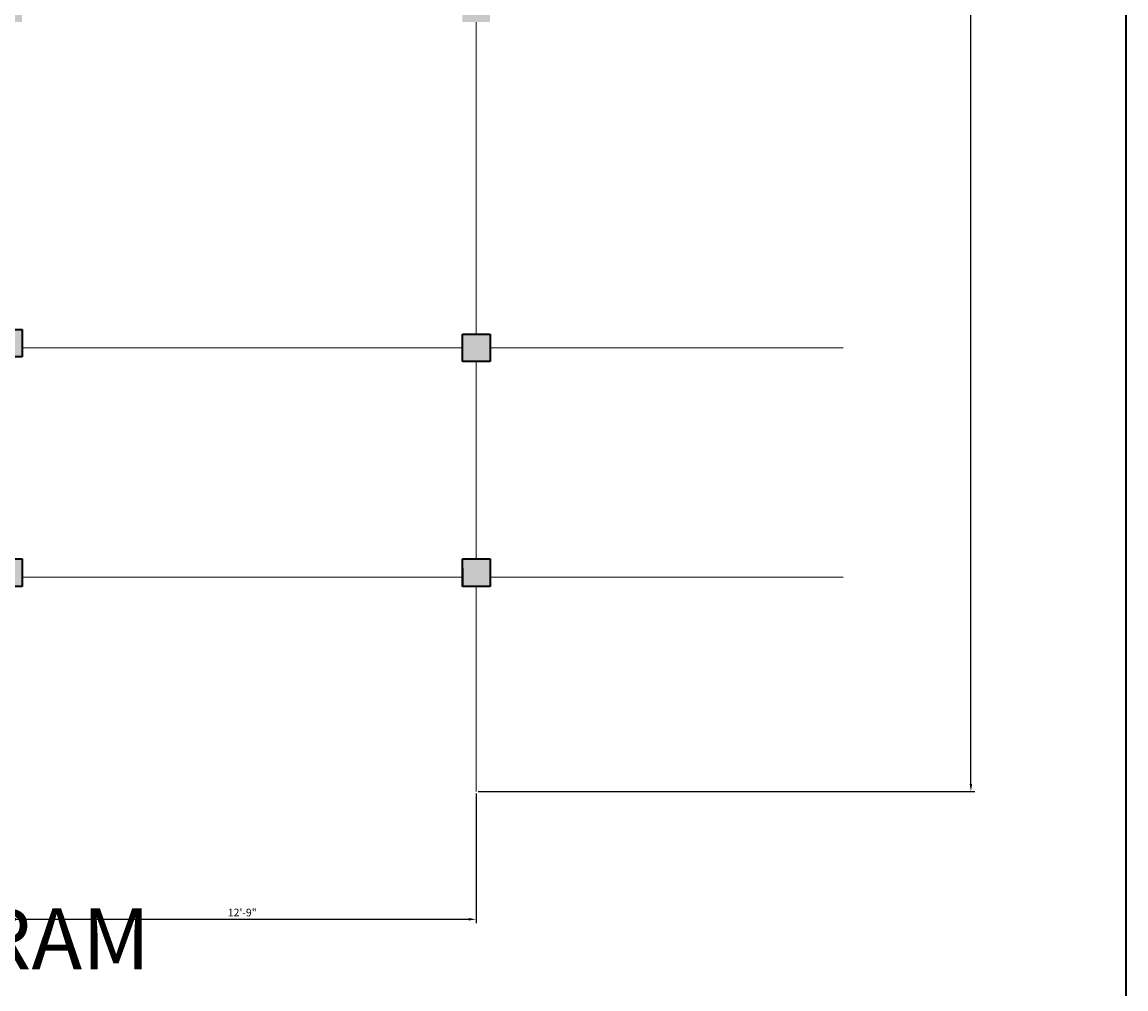
# Model space of a CAD drawing. Units: inches. Extents: x 6038 to 7543, y 3772 to 5131.
# Tile 11 of 14: x 7182 to 7543, y 4231 to 4547. Entities that reach past the tile are written whole.
import ezdxf

# ---------------------------------------------------------------- set-up
doc = ezdxf.new("R2010")
doc.units = ezdxf.units.IN
for name, color, linetype, lineweight in [('A-ANNO-DIMS', 4, 'Continuous', 18), ('A-ANNO-TITL', 3, 'Continuous', 30), ('A-ANNO-TTLB', 1, 'Continuous', 35), ('S-COLS', 7, 'Continuous', 35), ('S-COLS-PATT', 9, 'Continuous', 13), ('S-GRID', 6, 'Continuous', 13)]:
    doc.layers.add(name, color=color, linetype=linetype, lineweight=lineweight)
doc.styles.get("Standard").update_dxf_attribs({"font": 'arial.ttf'})
doc.dimstyles.new('ISO-25', dxfattribs={"dimtxt": 2.5, "dimasz": 2.5, "dimexe": 1.25, "dimexo": 0.625, "dimtad": 1, "dimdec": 0, "dimlunit": 3, "dimtxsty": 'Standard', "dimcen": 2.5, "dimadec": 0, "dimazin": 0, "dimtfac": 1, "dimtdec": 0, "dimtmove": 0, "dimatfit": 3, "dimfxl": 1, "dimarcsym": 0})

# ---------------------------------------------------------------- blocks, each defined once
blk = doc.blocks.new('COL-9X9')
for p, q in [((0, 9), (9, 9)), ((0, 0), (0, 9)), ((9, 9), (9, 0)), ((9, 0), (0, 0))]:
    blk.add_line(p, q)
blk = doc.blocks.new('*D86')
at = {"layer": 'A-ANNO-DIMS', "color": 0, "lineweight": -2, "transparency": 16777216}
for p, q in [((7177.09, 4294.9), (7177.09, 4252.53)), ((7330.09, 4294.9), (7330.09, 4252.53)), ((7179.59, 4253.78), (7327.59, 4253.78))]:
    blk.add_line(p, q, dxfattribs=at)
at = {"layer": 'A-ANNO-DIMS', "color": 0, "transparency": 16777216}
for points in [[(7179.59, 4254.2), (7179.59, 4253.36), (7177.09, 4253.78)], [(7327.59, 4254.2), (7327.59, 4253.36), (7330.09, 4253.78)]]:
    blk.add_solid(points, dxfattribs=at)
at = {"layer": 'Defpoints', "color": 0, "transparency": 16777216}
for p in [(7177.09, 4295.53), (7330.09, 4295.53), (7330.09, 4253.78)]:
    blk.add_point(p, dxfattribs=at)
at = {"layer": 'A-ANNO-DIMS', "color": 0, "transparency": 16777216, "insert": (7253.59, 4255.68), "char_height": 2.5, "attachment_point": 5}
blk.add_mtext('12\'-9"', dxfattribs=at)
blk = doc.blocks.new('*D93')
at = {"layer": 'A-ANNO-DIMS', "color": 0, "lineweight": -2, "transparency": 16777216}
for p, q in [((7330.71, 5049.84), (7493.09, 5049.84)), ((7491.84, 4298.03), (7491.84, 5047.34)), ((7330.71, 4295.53), (7493.09, 4295.53))]:
    blk.add_line(p, q, dxfattribs=at)
at = {"layer": 'A-ANNO-DIMS', "color": 0, "transparency": 16777216}
for points in [[(7491.43, 5047.34), (7492.26, 5047.34), (7491.84, 5049.84)], [(7491.43, 4298.03), (7492.26, 4298.03), (7491.84, 4295.53)]]:
    blk.add_solid(points, dxfattribs=at)
at = {"layer": 'Defpoints', "color": 0, "transparency": 16777216}
for p in [(7330.09, 5049.84), (7491.84, 5049.84), (7330.09, 4295.53)]:
    blk.add_point(p, dxfattribs=at)
at = {"layer": 'A-ANNO-DIMS', "color": 0, "transparency": 16777216, "insert": (7489.92, 4672.68), "char_height": 2.5, "attachment_point": 5, "rotation": 90}
blk.add_mtext('62\'-10 1/2"', dxfattribs=at)

msp = doc.modelspace()

# ---------------------------------------------------------------- hatches: boundary and pattern name
at = {"layer": 'S-COLS-PATT'}
h = msp.add_hatch(color=256, dxfattribs=at)
h.dxf.hatch_style = 1
h.paths.add_polyline_path([(7325.59, 4944.62), (7334.59, 4944.62), (7334.59, 4956.62), (7325.59, 4956.62)])
h.paths.add_polyline_path([(7334.59, 4746.62), (7334.59, 4758.62), (7325.59, 4758.62), (7325.59, 4746.62)])
h.paths.add_polyline_path([(7181.59, 4758.62), (7172.59, 4758.62), (7172.59, 4746.62), (7181.59, 4746.62)])
h.paths.add_polyline_path([(6983.59, 4758.62), (6974.59, 4758.62), (6974.59, 4746.62), (6983.59, 4746.62)])
h.paths.add_polyline_path([(6983.59, 4559.12), (6974.59, 4559.12), (6974.59, 4547.12), (6983.59, 4547.12)])
h.paths.add_polyline_path([(7181.59, 4559.12), (7172.59, 4559.12), (7172.59, 4547.12), (7181.59, 4547.12)])
h.paths.add_polyline_path([(7334.59, 4559.12), (7325.59, 4559.12), (7325.59, 4547.12), (7334.59, 4547.12)])
h = msp.add_hatch(color=256, dxfattribs=at)
h.dxf.hatch_style = 1
h.paths.add_polyline_path([(6974.59, 4884.62), (6983.59, 4884.62), (6983.59, 4893.62), (6974.59, 4893.62)])
h.paths.add_polyline_path([(7181.59, 4893.62), (7172.59, 4893.62), (7172.59, 4884.62), (7181.59, 4884.62)])
h.paths.add_polyline_path([(6983.59, 4436.12), (6983.59, 4445.12), (6974.59, 4445.12), (6974.59, 4436.12)])
h.paths.add_polyline_path([(7181.59, 4446.62), (7172.59, 4446.62), (7172.59, 4437.62), (7181.59, 4437.62)])
h.paths.add_polyline_path([(7325.59, 4436.12), (7334.59, 4436.12), (7334.59, 4445.12), (7325.59, 4445.12)])
h.paths.add_polyline_path([(7334.59, 4371.62), (7325.59, 4371.62), (7325.59, 4362.62), (7334.59, 4362.62)])
h.paths.add_polyline_path([(7181.59, 4362.62), (7181.59, 4371.62), (7172.59, 4371.62), (7172.59, 4362.62)])
h.paths.add_polyline_path([(6974.59, 4362.62), (6983.59, 4362.62), (6983.59, 4371.62), (6974.59, 4371.62)])

# ---------------------------------------------------------------- linework, layer by layer
at = {"layer": 'A-ANNO-TTLB'}
msp.add_lwpolyline([(6037.83, 5130.86), (7542.53, 5130.86), (7542.53, 3772.09), (6037.83, 3772.09)], close=True, dxfattribs=at)
at = {"layer": 'S-COLS'}
for p, q in [((7325.59, 4437.62), (7325.59, 4443.62)), ((7325.59, 4368.62), (7325.59, 4362.62))]:
    msp.add_line(p, q, dxfattribs=at)
at = {"layer": 'S-GRID'}
for p, q in [((7330.09, 4547.12), (7330.09, 4445.12)), ((7325.59, 4440.62), (7181.59, 4440.62)), ((7450.09, 4440.62), (7334.59, 4440.62)), ((7330.09, 4436.12), (7330.09, 4371.62)), ((7325.59, 4365.62), (7181.59, 4365.62)), ((7450.09, 4365.62), (7334.59, 4365.62)), ((7330.09, 4362.62), (7330.09, 4295.53))]:
    msp.add_line(p, q, dxfattribs=at)

# ---------------------------------------------------------------- block references
at = {"layer": 'S-COLS'}
for p in [(7172.59, 4437.62), (7325.59, 4436.12), (7172.59, 4362.62), (7325.59, 4362.62)]:
    msp.add_blockref('COL-9X9', p, dxfattribs=at)

# ---------------------------------------------------------------- texts
at = {"layer": 'A-ANNO-TITL', "insert": (6931.39, 4257.37), "char_height": 20, "attachment_point": 1}
msp.add_mtext_dynamic_manual_height_columns('CENTRE LINE DIAGRAM', width=549.9641, gutter_width=12.5, heights=[0], dxfattribs=at)

# ---------------------------------------------------------------- dimensions: what is measured, and where the dimension line sits
at = {"layer": 'A-ANNO-DIMS'}
dim = msp.add_linear_dim(base=(7491.84, 5049.84), p1=(7330.09, 4295.53), p2=(7330.09, 5049.84), angle=90, dimstyle='ISO-25', override={"dimdec": 1, "dimlfac": 1, "dimrnd": 0, "dimzin": 1, "dimdsep": 46, "dimlunit": 4, "dimfrac": 2}, dxfattribs=at)
dim.commit()
dim.dimension.update_dxf_attribs({"geometry": '*D93', "text_midpoint": (7489.92, 4672.68)})
dim = msp.add_linear_dim(base=(7330.09, 4253.78), p1=(7177.09, 4295.53), p2=(7330.09, 4295.53), dimstyle='ISO-25', override={"dimdec": 1, "dimlfac": 1, "dimrnd": 0, "dimzin": 1, "dimdsep": 46, "dimlunit": 4, "dimfrac": 2}, dxfattribs=at)
dim.commit()
dim.dimension.update_dxf_attribs({"geometry": '*D86', "text_midpoint": (7253.59, 4255.68)})

doc.saveas('drawing.dxf')
